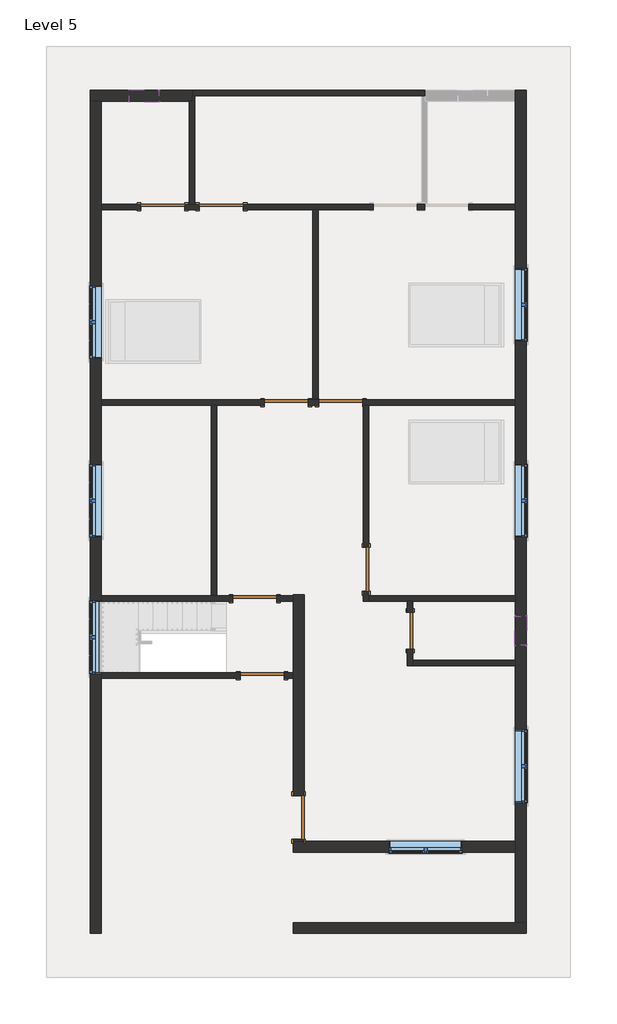
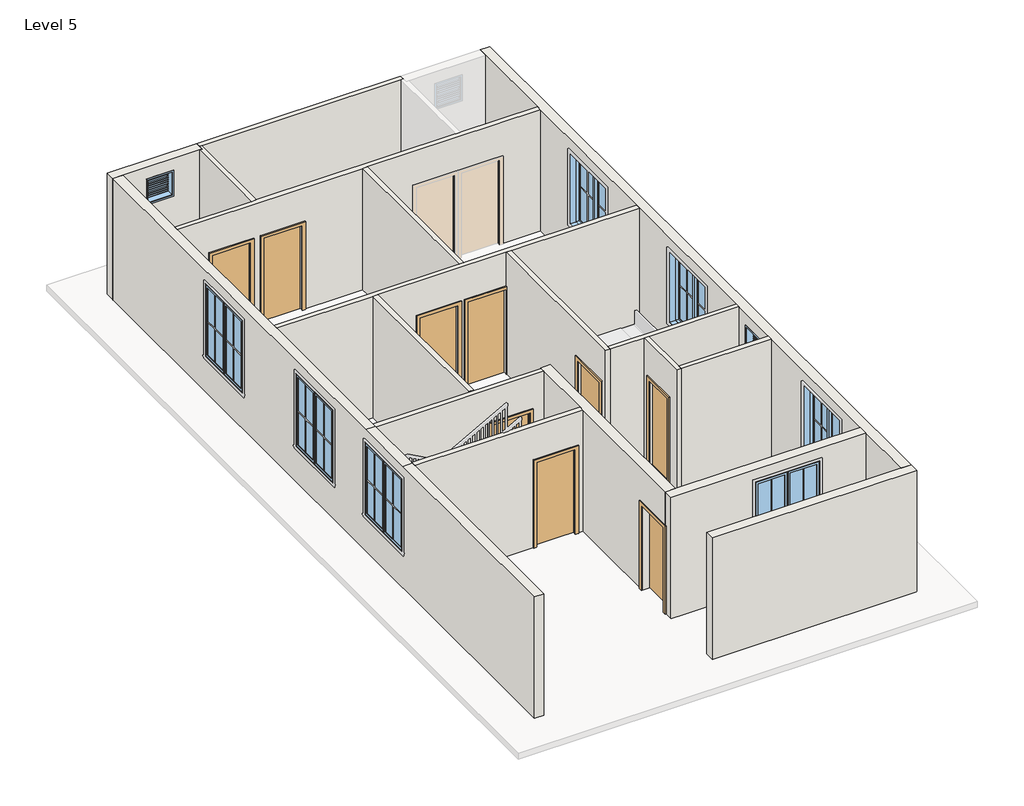
# One storey, part 1 of 3: 18 walls, 9 doors, 9 windows.
"""IFC4 building model written with IfcOpenShell, lengths in millimetres."""

from ifc_helpers import new_model, si_unit, frame, origin, place, context, project, spatial, polyline, outline, extrude, faceted_brep, transform, mapped, element, save
from components import door_78caadf7, single_flush_door_3_e5f9f3c4, single_flush_door_3_305aa2a5, single_flush_door_3_0ca8825f, window_casement_double_win_5_f93960c7, window_f2d8fef0

model = new_model("IFC4")

# Units and contexts
model_context = context("Model", 3, world=origin())
ifc_project = project(units=[si_unit("LENGTHUNIT", "METRE", prefix="MILLI")], contexts=[model_context])

# Site, building, storey
site = spatial("IfcSite", under=ifc_project)
building = spatial("IfcBuilding", under=site)
storey = spatial("IfcBuildingStorey", under=building, Name="Level 5", Elevation=9601.2)

# Doors
placement = place(None, origin())
door_shape = door_78caadf7(model_context)
element("IfcDoor", 1, ObjectType="Single-Flush : DOOR 2'6\"", at=placement, inside=storey, context=model_context, shape_type="MappedRepresentation", body=[
    mapped(door_shape, transform((860.2379845, -2779.6065691, 9601.2), x_axis=(0.0, 1.0, 0.0), y_axis=(-1.0, 0.0, 0.0), z_axis=(0.0, 0.0, 1.0))),
])
single_flush_door_3_shape = single_flush_door_3_e5f9f3c4(model_context)
element("IfcDoor", 2, ObjectType="Single-Flush : DOOR 3'", at=placement, inside=storey, context=model_context, shape_type="MappedRepresentation", body=[
    mapped(single_flush_door_3_shape, transform((-54.1620155, -1503.2565691, 9601.2), x_axis=(0.0, -1.0, 0.0), y_axis=(1.0, 0.0, 0.0), z_axis=(0.0, 0.0, 1.0))),
])
element("IfcDoor", 3, ObjectType="Single-Flush : DOOR 3'", at=placement, inside=storey, context=model_context, shape_type="MappedRepresentation", body=[
    mapped(single_flush_door_3_shape, transform((-1717.8620155, 1963.8434309, 9601.2), x_axis=(1.0, 0.0, 0.0), y_axis=(0.0, 1.0, 0.0), z_axis=(0.0, 0.0, 1.0))),
])
element("IfcDoor", 4, ObjectType="Single-Flush : DOOR 3'", at=placement, inside=storey, context=model_context, shape_type="MappedRepresentation", body=[
    mapped(single_flush_door_3_shape, transform((-2371.9120155, -2112.8565691, 9601.2), x_axis=(1.0, 0.0, 0.0), y_axis=(0.0, 1.0, 0.0), z_axis=(0.0, 0.0, 1.0))),
])
element("IfcDoor", 5, ObjectType="Single-Flush : DOOR 3'", at=placement, inside=storey, context=model_context, shape_type="MappedRepresentation", body=[
    mapped(single_flush_door_3_shape, transform((-2219.5120155, -3713.0565691, 9601.2), x_axis=(1.0, 0.0, 0.0), y_axis=(0.0, 1.0, 0.0), z_axis=(0.0, 0.0, 1.0))),
])
element("IfcDoor", 6, ObjectType="Single-Flush : DOOR 3'", at=placement, inside=storey, context=model_context, shape_type="MappedRepresentation", body=[
    mapped(single_flush_door_3_shape, transform((-4283.2620155, 6040.5434309, 9601.2), x_axis=(1.0, 0.0, 0.0), y_axis=(0.0, 1.0, 0.0), z_axis=(0.0, 0.0, 1.0))),
])
single_flush_door_3_2_shape = single_flush_door_3_305aa2a5(model_context)
element("IfcDoor", 7, ObjectType="Single-Flush : DOOR 3'", at=placement, inside=storey, context=model_context, shape_type="MappedRepresentation", body=[
    mapped(single_flush_door_3_2_shape, transform((-581.2120155, 1963.8434309, 9601.2), x_axis=(-1.0, 0.0, 0.0), y_axis=(0.0, -1.0, 0.0), z_axis=(0.0, 0.0, 1.0))),
])
element("IfcDoor", 8, ObjectType="Single-Flush : DOOR 3'", at=placement, inside=storey, context=model_context, shape_type="MappedRepresentation", body=[
    mapped(single_flush_door_3_2_shape, transform((-3064.0620155, 6040.5434309, 9601.2), x_axis=(-1.0, 0.0, 0.0), y_axis=(0.0, -1.0, 0.0), z_axis=(0.0, 0.0, 1.0))),
])
single_flush_door_3_3_shape = single_flush_door_3_0ca8825f(model_context)
element("IfcDoor", 9, ObjectType="Single-Flush : DOOR 3'", at=placement, inside=storey, context=model_context, shape_type="MappedRepresentation", body=[
    mapped(single_flush_door_3_3_shape, transform((-1457.5120155, -6665.8065691, 9601.2), x_axis=(0.0, -1.0, 0.0), y_axis=(1.0, 0.0, 0.0), z_axis=(0.0, 0.0, 1.0))),
])

# Walls
element("IfcWall", 10, ObjectType="WALL 4.5\"", at=placement, inside=storey, context=model_context, shape_type="Brep", body=[
    faceted_brep([(-3673.6620155, 8345.5934309, 9601.2), (-3616.5120155, 8345.5934309, 9601.2), (1107.8879845, 8345.5934309, 9601.2), (1165.0379845, 8345.5934309, 9601.2), (1165.0379845, 8345.5934309, 12649.2), (1107.8879845, 8345.5934309, 12649.2), (-3616.5120155, 8345.5934309, 12649.2), (-3673.6620155, 8345.5934309, 12649.2), (-3673.6620155, 8459.8934309, 9601.2), (-3673.6620155, 8459.8934309, 12649.2), (1165.0379845, 8459.8934309, 12649.2), (1165.0379845, 8459.8934309, 9601.2)], [[[0, 1, 2, 3, 4, 5, 6, 7]], [[8, 9, 10, 11]], [[3, 2, 1, 0, 8, 11]], [[4, 3, 11, 10]], [[0, 7, 9, 8]], [[7, 6, 5, 4, 10, 9]]]),
])
element("IfcWall", 11, ObjectType="WALL 4.5\"", at=placement, inside=storey, context=model_context, shape_type="SweptSolid", body=[
    extrude(outline(polyline([(-3730.8120155, 6097.6934309), (-3730.8120155, 8231.2934309), (-3673.6620155, 8231.2934309), (-3673.6620155, 8345.5934309), (-3616.5120155, 8345.5934309), (-3616.5120155, 6097.6934309), (-3730.8120155, 6097.6934309)])), frame((0.0, 0.0, 9601.2), z_axis=(0.0, 0.0, 1.0), x_axis=(1.0, 0.0, 0.0)), (0.0, 0.0, 1.0), 3048.0),
])
element("IfcWall", 12, ObjectType="WALL 4.5\"", at=placement, inside=storey, context=model_context, shape_type="Brep", body=[
    faceted_brep([(1165.0379845, 6097.6934309, 11734.8), (1165.0379845, 6097.6934309, 9601.2), (1107.8879845, 6097.6934309, 9601.2), (1012.6379845, 6097.6934309, 9601.2), (1012.6379845, 6097.6934309, 11734.8), (98.2379845, 6097.6934309, 11734.8), (98.2379845, 6097.6934309, 9601.2), (-2606.8620155, 6097.6934309, 9601.2), (-2606.8620155, 6097.6934309, 11734.8), (-3521.2620155, 6097.6934309, 11734.8), (-3521.2620155, 6097.6934309, 9601.2), (-3616.5120155, 6097.6934309, 9601.2), (-3730.8120155, 6097.6934309, 9601.2), (-3826.0620155, 6097.6934309, 9601.2), (-3826.0620155, 6097.6934309, 11734.8), (-4740.4620155, 6097.6934309, 11734.8), (-4740.4620155, 6097.6934309, 9601.2), (-5559.6120155, 6097.6934309, 9601.2), (-5559.6120155, 6097.6934309, 12649.2), (-3730.8120155, 6097.6934309, 12649.2), (-3616.5120155, 6097.6934309, 12649.2), (1107.8879845, 6097.6934309, 12649.2), (1222.1879845, 6097.6934309, 12649.2), (3050.9879845, 6097.6934309, 12649.2), (3050.9879845, 6097.6934309, 9601.2), (2079.4379845, 6097.6934309, 9601.2), (2079.4379845, 6097.6934309, 11734.8), (1012.6379845, 5983.3934309, 9601.2), (1165.0379845, 5983.3934309, 9601.2), (1165.0379845, 5983.3934309, 11734.8), (2079.4379845, 5983.3934309, 11734.8), (2079.4379845, 5983.3934309, 9601.2), (3050.9879845, 5983.3934309, 9601.2), (3050.9879845, 5983.3934309, 12649.2), (-1051.1120155, 5983.3934309, 12649.2), (-1165.4120155, 5983.3934309, 12649.2), (-5559.6120155, 5983.3934309, 12649.2), (-5559.6120155, 5983.3934309, 9601.2), (-4740.4620155, 5983.3934309, 9601.2), (-4740.4620155, 5983.3934309, 11734.8), (-3826.0620155, 5983.3934309, 11734.8), (-3826.0620155, 5983.3934309, 9601.2), (-3521.2620155, 5983.3934309, 9601.2), (-3521.2620155, 5983.3934309, 11734.8), (-2606.8620155, 5983.3934309, 11734.8), (-2606.8620155, 5983.3934309, 9601.2), (-1165.4120155, 5983.3934309, 9601.2), (-1051.1120155, 5983.3934309, 9601.2), (98.2379845, 5983.3934309, 9601.2), (98.2379845, 5983.3934309, 11734.8), (1012.6379845, 5983.3934309, 11734.8)], [[[0, 1, 2, 3, 4, 5, 6, 7, 8, 9, 10, 11, 12, 13, 14, 15, 16, 17, 18, 19, 20, 21, 22, 23, 24, 25, 26]], [[27, 28, 29, 30, 31, 32, 33, 34, 35, 36, 37, 38, 39, 40, 41, 42, 43, 44, 45, 46, 47, 48, 49, 50]], [[38, 37, 17, 16]], [[13, 12, 11, 10, 42, 41]], [[48, 47, 46, 45, 7, 6]], [[25, 24, 32, 31]], [[3, 2, 1, 28, 27]], [[18, 17, 37, 36]], [[24, 23, 33, 32]], [[14, 13, 41, 40]], [[15, 14, 40, 39]], [[16, 15, 39, 38]], [[43, 42, 10, 9]], [[44, 43, 9, 8]], [[45, 44, 8, 7]], [[4, 3, 27, 50]], [[5, 4, 50, 49]], [[6, 5, 49, 48]], [[29, 28, 1, 0]], [[30, 29, 0, 26]], [[31, 30, 26, 25]], [[23, 22, 21, 20, 19, 18, 36, 35, 34, 33]]]),
])
element("IfcWall", 13, ObjectType="WALL 4.5\"", at=placement, inside=storey, context=model_context, shape_type="SweptSolid", body=[
    extrude(outline(polyline([(-1165.4120155, 2020.9934309), (-1165.4120155, 5983.3934309), (-1051.1120155, 5983.3934309), (-1051.1120155, 2020.9934309), (-1165.4120155, 2020.9934309)])), frame((0.0, 0.0, 9601.2), z_axis=(0.0, 0.0, 1.0), x_axis=(1.0, 0.0, 0.0)), (0.0, 0.0, 1.0), 3048.0),
])
element("IfcWall", 14, ObjectType="WALL 4.5\"", at=placement, inside=storey, context=model_context, shape_type="Brep", body=[
    faceted_brep([(-1260.6620155, 1906.6934309, 11734.8), (-1260.6620155, 1906.6934309, 9601.2), (-1038.4120155, 1906.6934309, 9601.2), (-1038.4120155, 1906.6934309, 11734.8), (-124.0120155, 1906.6934309, 11734.8), (-124.0120155, 1906.6934309, 9601.2), (-111.3120155, 1906.6934309, 9601.2), (2.9879845, 1906.6934309, 9601.2), (3050.9879845, 1906.6934309, 9601.2), (3050.9879845, 1906.6934309, 12649.2), (2.9879845, 1906.6934309, 12649.2), (-111.3120155, 1906.6934309, 12649.2), (-3159.3120155, 1906.6934309, 12649.2), (-3273.6120155, 1906.6934309, 12649.2), (-5559.6120155, 1906.6934309, 12649.2), (-5559.6120155, 1906.6934309, 9601.2), (-3273.6120155, 1906.6934309, 9601.2), (-3159.3120155, 1906.6934309, 9601.2), (-2175.0620155, 1906.6934309, 9601.2), (-2175.0620155, 1906.6934309, 11734.8), (-1038.4120155, 2020.9934309, 9601.2), (-1051.1120155, 2020.9934309, 9601.2), (-1165.4120155, 2020.9934309, 9601.2), (-1260.6620155, 2020.9934309, 9601.2), (-1260.6620155, 2020.9934309, 11734.8), (-2175.0620155, 2020.9934309, 11734.8), (-2175.0620155, 2020.9934309, 9601.2), (-5559.6120155, 2020.9934309, 9601.2), (-5559.6120155, 2020.9934309, 12649.2), (-1165.4120155, 2020.9934309, 12649.2), (-1051.1120155, 2020.9934309, 12649.2), (3050.9879845, 2020.9934309, 12649.2), (3050.9879845, 2020.9934309, 9601.2), (-124.0120155, 2020.9934309, 9601.2), (-124.0120155, 2020.9934309, 11734.8), (-1038.4120155, 2020.9934309, 11734.8)], [[[0, 1, 2, 3, 4, 5, 6, 7, 8, 9, 10, 11, 12, 13, 14, 15, 16, 17, 18, 19]], [[20, 21, 22, 23, 24, 25, 26, 27, 28, 29, 30, 31, 32, 33, 34, 35]], [[33, 32, 8, 7, 6, 5]], [[2, 1, 23, 22, 21, 20]], [[18, 17, 16, 15, 27, 26]], [[15, 14, 28, 27]], [[9, 8, 32, 31]], [[3, 2, 20, 35]], [[4, 3, 35, 34]], [[5, 4, 34, 33]], [[24, 23, 1, 0]], [[25, 24, 0, 19]], [[26, 25, 19, 18]], [[14, 13, 12, 11, 10, 9, 31, 30, 29, 28]]]),
])
element("IfcWall", 15, ObjectType="WALL 4.5\"", at=placement, inside=storey, context=model_context, shape_type="SweptSolid", body=[
    extrude(outline(polyline([(-3273.6120155, -2032.8465691), (-3273.6120155, 1906.6934309), (-3159.3120155, 1906.6934309), (-3159.3120155, -2032.8465691), (-3273.6120155, -2032.8465691)])), frame((0.0, 0.0, 9601.2), z_axis=(0.0, 0.0, 1.0), x_axis=(1.0, 0.0, 0.0)), (0.0, 0.0, 1.0), 3048.0),
])
element("IfcWall", 16, ObjectType="WALL 4.5\"", at=placement, inside=storey, context=model_context, shape_type="SweptSolid", body=[
    extrude(outline(polyline([(11734.8, -1914.7120155), (9601.2, -1914.7120155), (9601.2, -1571.8120155), (12649.2, -1571.8120155), (12649.2, -5559.6120155), (9601.2, -5559.6120155), (9601.2, -2829.1120155), (11734.8, -2829.1120155), (11734.8, -1914.7120155)])), frame((0.0, -2170.0065691, 0.0), z_axis=(0.0, 1.0, 0.0), x_axis=(0.0, 0.0, 1.0)), (0.0, 0.0, 1.0), 114.3),
])
element("IfcWall", 17, ObjectType="WALL 4.5\"", at=placement, inside=storey, context=model_context, shape_type="SweptSolid", body=[
    extrude(outline(polyline([(11734.8, -1762.3120155), (9601.2, -1762.3120155), (9601.2, -1571.8120155), (12649.2, -1571.8120155), (12649.2, -5559.6120155), (9601.2, -5559.6120155), (9601.2, -2676.7120155), (11734.8, -2676.7120155), (11734.8, -1762.3120155)])), frame((0.0, -3770.2065691, 0.0), z_axis=(0.0, 1.0, 0.0), x_axis=(0.0, 0.0, 1.0)), (0.0, 0.0, 1.0), 114.3),
])
element("IfcWall", 18, ObjectType="WALL 4.5\"", at=placement, inside=storey, context=model_context, shape_type="Brep", body=[
    faceted_brep([(-111.3120155, -1960.4565691, 11734.8), (-111.3120155, -1960.4565691, 9601.2), (-111.3120155, -2170.0065691, 9601.2), (-111.3120155, -2170.0065691, 12649.2), (-111.3120155, 1906.6934309, 12649.2), (-111.3120155, 1906.6934309, 9601.2), (-111.3120155, -1046.0565691, 9601.2), (-111.3120155, -1046.0565691, 11734.8), (2.9879845, -2170.0065691, 9601.2), (2.9879845, -2055.7065691, 9601.2), (2.9879845, -1960.4565691, 9601.2), (2.9879845, -1960.4565691, 11734.8), (2.9879845, -1046.0565691, 11734.8), (2.9879845, -1046.0565691, 9601.2), (2.9879845, 1906.6934309, 9601.2), (2.9879845, 1906.6934309, 12649.2), (2.9879845, -2055.7065691, 12649.2), (2.9879845, -2170.0065691, 12649.2)], [[[0, 1, 2, 3, 4, 5, 6, 7]], [[8, 9, 10, 11, 12, 13, 14, 15, 16, 17]], [[6, 5, 14, 13]], [[2, 1, 10, 9, 8]], [[5, 4, 15, 14]], [[3, 2, 8, 17]], [[11, 10, 1, 0]], [[12, 11, 0, 7]], [[13, 12, 7, 6]], [[4, 3, 17, 16, 15]]]),
])
element("IfcWall", 19, ObjectType="WALL 4.5\"", at=placement, inside=storey, context=model_context, shape_type="Brep", body=[
    faceted_brep([(2.9879845, -2170.0065691, 9601.2), (803.0879845, -2170.0065691, 9601.2), (917.3879845, -2170.0065691, 9601.2), (3050.9879845, -2170.0065691, 9601.2), (3050.9879845, -2170.0065691, 12649.2), (917.3879845, -2170.0065691, 12649.2), (803.0879845, -2170.0065691, 12649.2), (2.9879845, -2170.0065691, 12649.2), (2.9879845, -2055.7065691, 9601.2), (2.9879845, -2055.7065691, 12649.2), (3050.9879845, -2055.7065691, 12649.2), (3050.9879845, -2055.7065691, 9601.2)], [[[0, 1, 2, 3, 4, 5, 6, 7]], [[8, 9, 10, 11]], [[3, 2, 1, 0, 8, 11]], [[0, 7, 9, 8]], [[4, 3, 11, 10]], [[7, 6, 5, 4, 10, 9]]]),
])
element("IfcWall", 20, ObjectType="WALL 4.5\"", at=placement, inside=storey, context=model_context, shape_type="Brep", body=[
    faceted_brep([(803.0879845, -2170.0065691, 9601.2), (803.0879845, -2398.6065691, 9601.2), (803.0879845, -2398.6065691, 11734.8), (803.0879845, -3160.6065691, 11734.8), (803.0879845, -3160.6065691, 9601.2), (803.0879845, -3503.5065691, 9601.2), (803.0879845, -3503.5065691, 12649.2), (803.0879845, -2170.0065691, 12649.2), (917.3879845, -2398.6065691, 11734.8), (917.3879845, -2398.6065691, 9601.2), (917.3879845, -2170.0065691, 9601.2), (917.3879845, -2170.0065691, 12649.2), (917.3879845, -3389.2065691, 12649.2), (917.3879845, -3503.5065691, 12649.2), (917.3879845, -3503.5065691, 9601.2), (917.3879845, -3389.2065691, 9601.2), (917.3879845, -3160.6065691, 9601.2), (917.3879845, -3160.6065691, 11734.8)], [[[0, 1, 2, 3, 4, 5, 6, 7]], [[8, 9, 10, 11, 12, 13, 14, 15, 16, 17]], [[10, 9, 1, 0]], [[16, 15, 14, 5, 4]], [[0, 7, 11, 10]], [[6, 5, 14, 13]], [[2, 1, 9, 8]], [[3, 2, 8, 17]], [[4, 3, 17, 16]], [[7, 6, 13, 12, 11]]]),
])
element("IfcWall", 21, ObjectType="WALL 4.5\"", at=placement, inside=storey, context=model_context, shape_type="SweptSolid", body=[
    extrude(outline(polyline([(917.3879845, -3389.2065691), (3050.9879845, -3389.2065691), (3050.9879845, -3503.5065691), (917.3879845, -3503.5065691), (917.3879845, -3389.2065691)])), frame((0.0, 0.0, 9601.2), z_axis=(0.0, 0.0, 1.0), x_axis=(1.0, 0.0, 0.0)), (0.0, 0.0, 1.0), 3048.0),
])
element("IfcWall", 22, ObjectType="WALL 9\"", at=placement, inside=storey, context=model_context, shape_type="Brep", body=[
    faceted_brep([(-3673.6620155, 8459.8934309, 9601.2), (-5788.2120155, 8459.8934309, 9601.2), (-5788.2120155, 8459.8934309, 12649.2), (-3673.6620155, 8459.8934309, 12649.2), (-4978.5870155, 8459.8934309, 12344.4), (-4978.5870155, 8459.8934309, 11734.8), (-4368.9870155, 8459.8934309, 11734.8), (-4368.9870155, 8459.8934309, 12344.4), (-3673.6620155, 8231.2934309, 9601.2), (-3673.6620155, 8231.2934309, 12649.2), (-3730.8120155, 8231.2934309, 12649.2), (-5559.6120155, 8231.2934309, 12649.2), (-5788.2120155, 8231.2934309, 12649.2), (-5788.2120155, 8231.2934309, 9601.2), (-5559.6120155, 8231.2934309, 9601.2), (-3730.8120155, 8231.2934309, 9601.2), (-4978.5870155, 8231.2934309, 12344.4), (-4368.9870155, 8231.2934309, 12344.4), (-4368.9870155, 8231.2934309, 11734.8), (-4978.5870155, 8231.2934309, 11734.8), (-3673.6620155, 8345.5934309, 9601.2), (-3673.6620155, 8345.5934309, 12649.2)], [[[0, 1, 2, 3], [4, 5, 6, 7]], [[8, 9, 10, 11, 12, 13, 14, 15], [16, 17, 18, 19]], [[1, 0, 20, 8, 15, 14, 13]], [[0, 3, 21, 9, 8, 20]], [[2, 1, 13, 12]], [[5, 4, 16, 19]], [[6, 5, 19, 18]], [[7, 6, 18, 17]], [[4, 7, 17, 16]], [[3, 2, 12, 11, 10, 9, 21]]]),
])
element("IfcWall", 23, ObjectType="WALL 9\"", at=placement, inside=storey, context=model_context, shape_type="Brep", body=[
    faceted_brep([(-5788.2120155, 8231.2934309, 9601.2), (-5788.2120155, -9078.8065691, 9601.2), (-5788.2120155, -9078.8065691, 12649.2), (-5788.2120155, -3674.9565691, 12649.2), (-5788.2120155, -2150.9565691, 12649.2), (-5788.2120155, 8231.2934309, 12649.2), (-5788.2120155, 4402.2434309, 12344.4), (-5788.2120155, 2878.2434309, 12344.4), (-5788.2120155, 2878.2434309, 10515.6), (-5788.2120155, 4402.2434309, 10515.6), (-5788.2120155, -2150.9565691, 12344.4), (-5788.2120155, -3674.9565691, 12344.4), (-5788.2120155, -3674.9565691, 10515.6), (-5788.2120155, -2150.9565691, 10515.6), (-5788.2120155, 687.4934309, 12344.4), (-5788.2120155, -836.5065691, 12344.4), (-5788.2120155, -836.5065691, 10515.6), (-5788.2120155, 687.4934309, 10515.6), (-5559.6120155, 8231.2934309, 9601.2), (-5559.6120155, 8231.2934309, 12649.2), (-5559.6120155, 6097.6934309, 12649.2), (-5559.6120155, 5983.3934309, 12649.2), (-5559.6120155, 2020.9934309, 12649.2), (-5559.6120155, 1906.6934309, 12649.2), (-5559.6120155, -2055.7065691, 12649.2), (-5559.6120155, -2150.9565691, 12649.2), (-5559.6120155, -2170.0065691, 12649.2), (-5559.6120155, -3655.9065691, 12649.2), (-5559.6120155, -3674.9565691, 12649.2), (-5559.6120155, -3770.2065691, 12649.2), (-5559.6120155, -9078.8065691, 12649.2), (-5559.6120155, -9078.8065691, 9601.2), (-5559.6120155, -3770.2065691, 9601.2), (-5559.6120155, -3655.9065691, 9601.2), (-5559.6120155, -2170.0065691, 9601.2), (-5559.6120155, -2055.7065691, 9601.2), (-5559.6120155, 1906.6934309, 9601.2), (-5559.6120155, 2020.9934309, 9601.2), (-5559.6120155, 5983.3934309, 9601.2), (-5559.6120155, 6097.6934309, 9601.2), (-5559.6120155, 4402.2434309, 12344.4), (-5559.6120155, 4402.2434309, 10515.6), (-5559.6120155, 2878.2434309, 10515.6), (-5559.6120155, 2878.2434309, 12344.4), (-5559.6120155, -2150.9565691, 12344.4), (-5559.6120155, -2150.9565691, 10515.6), (-5559.6120155, -3674.9565691, 10515.6), (-5559.6120155, -3674.9565691, 12344.4), (-5559.6120155, 687.4934309, 12344.4), (-5559.6120155, 687.4934309, 10515.6), (-5559.6120155, -836.5065691, 10515.6), (-5559.6120155, -836.5065691, 12344.4)], [[[0, 1, 2, 3, 4, 5], [6, 7, 8, 9], [10, 11, 12, 13], [14, 15, 16, 17]], [[18, 19, 20, 21, 22, 23, 24, 25, 26, 27, 28, 29, 30, 31, 32, 33, 34, 35, 36, 37, 38, 39], [40, 41, 42, 43], [44, 45, 46, 47], [48, 49, 50, 51]], [[1, 0, 18, 39, 38, 37, 36, 35, 34, 33, 32, 31]], [[2, 1, 31, 30]], [[0, 5, 19, 18]], [[41, 40, 6, 9]], [[42, 41, 9, 8]], [[43, 42, 8, 7]], [[40, 43, 7, 6]], [[45, 44, 10, 13]], [[46, 45, 13, 12]], [[47, 46, 12, 11]], [[44, 47, 11, 10]], [[49, 48, 14, 17]], [[50, 49, 17, 16]], [[51, 50, 16, 15]], [[48, 51, 15, 14]], [[4, 3, 28, 27, 26, 25]], [[3, 2, 30, 29, 28]], [[5, 4, 25, 24, 23, 22, 21, 20, 19]]]),
])
element("IfcWall", 24, ObjectType="WALL 9\"", at=placement, inside=storey, context=model_context, shape_type="Brep", body=[
    faceted_brep([(-1571.8120155, -9078.8065691, 9601.2), (3279.5879845, -9078.8065691, 9601.2), (3279.5879845, -9078.8065691, 12649.2), (-1571.8120155, -9078.8065691, 12649.2), (-1571.8120155, -8850.2065691, 9601.2), (-1571.8120155, -8850.2065691, 12649.2), (3050.9879845, -8850.2065691, 12649.2), (3279.5879845, -8850.2065691, 12649.2), (3279.5879845, -8850.2065691, 9601.2), (3050.9879845, -8850.2065691, 9601.2)], [[[0, 1, 2, 3]], [[4, 5, 6, 7, 8, 9]], [[1, 0, 4, 9, 8]], [[0, 3, 5, 4]], [[2, 1, 8, 7]], [[3, 2, 7, 6, 5]]]),
])
element("IfcWall", 25, ObjectType="WALL 9\"", at=placement, inside=storey, context=model_context, shape_type="Brep", body=[
    faceted_brep([(3279.5879845, -8850.2065691, 9601.2), (3279.5879845, 8459.8934309, 9601.2), (3279.5879845, 8459.8934309, 12649.2), (3279.5879845, -8850.2065691, 12649.2), (3279.5879845, 3240.1934309, 12344.4), (3279.5879845, 4764.1934309, 12344.4), (3279.5879845, 4764.1934309, 10515.6), (3279.5879845, 3240.1934309, 10515.6), (3279.5879845, -836.5065691, 12344.4), (3279.5879845, 687.4934309, 12344.4), (3279.5879845, 687.4934309, 10515.6), (3279.5879845, -836.5065691, 10515.6), (3279.5879845, -6361.0065691, 12344.4), (3279.5879845, -4837.0065691, 12344.4), (3279.5879845, -4837.0065691, 10515.6), (3279.5879845, -6361.0065691, 10515.6), (3279.5879845, -2474.8065691, 12344.4), (3279.5879845, -2474.8065691, 11734.8), (3279.5879845, -3084.4065691, 11734.8), (3279.5879845, -3084.4065691, 12344.4), (3050.9879845, -8850.2065691, 9601.2), (3050.9879845, -8850.2065691, 12649.2), (3050.9879845, -7389.7065691, 12649.2), (3050.9879845, -7161.1065691, 12649.2), (3050.9879845, -3503.5065691, 12649.2), (3050.9879845, -3389.2065691, 12649.2), (3050.9879845, -2170.0065691, 12649.2), (3050.9879845, -2055.7065691, 12649.2), (3050.9879845, 1906.6934309, 12649.2), (3050.9879845, 2020.9934309, 12649.2), (3050.9879845, 5983.3934309, 12649.2), (3050.9879845, 6097.6934309, 12649.2), (3050.9879845, 8231.2934309, 12649.2), (3050.9879845, 8459.8934309, 12649.2), (3050.9879845, 8459.8934309, 9601.2), (3050.9879845, 8231.2934309, 9601.2), (3050.9879845, 6097.6934309, 9601.2), (3050.9879845, 5983.3934309, 9601.2), (3050.9879845, 2020.9934309, 9601.2), (3050.9879845, 1906.6934309, 9601.2), (3050.9879845, -2055.7065691, 9601.2), (3050.9879845, -2170.0065691, 9601.2), (3050.9879845, -3389.2065691, 9601.2), (3050.9879845, -3503.5065691, 9601.2), (3050.9879845, -7161.1065691, 9601.2), (3050.9879845, -7389.7065691, 9601.2), (3050.9879845, 3240.1934309, 12344.4), (3050.9879845, 3240.1934309, 10515.6), (3050.9879845, 4764.1934309, 10515.6), (3050.9879845, 4764.1934309, 12344.4), (3050.9879845, -836.5065691, 12344.4), (3050.9879845, -836.5065691, 10515.6), (3050.9879845, 687.4934309, 10515.6), (3050.9879845, 687.4934309, 12344.4), (3050.9879845, -6361.0065691, 12344.4), (3050.9879845, -6361.0065691, 10515.6), (3050.9879845, -4837.0065691, 10515.6), (3050.9879845, -4837.0065691, 12344.4), (3050.9879845, -2474.8065691, 12344.4), (3050.9879845, -3084.4065691, 12344.4), (3050.9879845, -3084.4065691, 11734.8), (3050.9879845, -2474.8065691, 11734.8)], [[[0, 1, 2, 3], [4, 5, 6, 7], [8, 9, 10, 11], [12, 13, 14, 15], [16, 17, 18, 19]], [[20, 21, 22, 23, 24, 25, 26, 27, 28, 29, 30, 31, 32, 33, 34, 35, 36, 37, 38, 39, 40, 41, 42, 43, 44, 45], [46, 47, 48, 49], [50, 51, 52, 53], [54, 55, 56, 57], [58, 59, 60, 61]], [[1, 0, 20, 45, 44, 43, 42, 41, 40, 39, 38, 37, 36, 35, 34]], [[0, 3, 21, 20]], [[2, 1, 34, 33]], [[47, 46, 4, 7]], [[48, 47, 7, 6]], [[49, 48, 6, 5]], [[46, 49, 5, 4]], [[51, 50, 8, 11]], [[52, 51, 11, 10]], [[53, 52, 10, 9]], [[50, 53, 9, 8]], [[55, 54, 12, 15]], [[56, 55, 15, 14]], [[57, 56, 14, 13]], [[54, 57, 13, 12]], [[17, 16, 58, 61]], [[18, 17, 61, 60]], [[19, 18, 60, 59]], [[16, 19, 59, 58]], [[3, 2, 33, 32, 31, 30, 29, 28, 27, 26, 25, 24, 23, 22, 21]]]),
])
element("IfcWall", 26, ObjectType="WALL 9\"", at=placement, inside=storey, context=model_context, shape_type="Brep", body=[
    faceted_brep([(3050.9879845, -7161.1065691, 9601.2), (-1343.2120155, -7161.1065691, 9601.2), (-1571.8120155, -7161.1065691, 9601.2), (-1571.8120155, -7161.1065691, 12649.2), (-1343.2120155, -7161.1065691, 12649.2), (3050.9879845, -7161.1065691, 12649.2), (422.0879845, -7161.1065691, 12344.4), (422.0879845, -7161.1065691, 10515.6), (1946.0879845, -7161.1065691, 10515.6), (1946.0879845, -7161.1065691, 12344.4), (3050.9879845, -7389.7065691, 9601.2), (3050.9879845, -7389.7065691, 12649.2), (-1571.8120155, -7389.7065691, 12649.2), (-1571.8120155, -7389.7065691, 9601.2), (422.0879845, -7389.7065691, 12344.4), (1946.0879845, -7389.7065691, 12344.4), (1946.0879845, -7389.7065691, 10515.6), (422.0879845, -7389.7065691, 10515.6)], [[[0, 1, 2, 3, 4, 5], [6, 7, 8, 9]], [[10, 11, 12, 13], [14, 15, 16, 17]], [[2, 1, 0, 10, 13]], [[0, 5, 11, 10]], [[3, 2, 13, 12]], [[7, 6, 14, 17]], [[8, 7, 17, 16]], [[9, 8, 16, 15]], [[6, 9, 15, 14]], [[5, 4, 3, 12, 11]]]),
])
element("IfcWall", 27, ObjectType="WALL 9\"", at=placement, inside=storey, context=model_context, shape_type="Brep", body=[
    faceted_brep([(-1343.2120155, -7161.1065691, 9601.2), (-1343.2120155, -7123.0065691, 9601.2), (-1343.2120155, -7123.0065691, 11734.8), (-1343.2120155, -6208.6065691, 11734.8), (-1343.2120155, -6208.6065691, 9601.2), (-1343.2120155, -2032.8465691, 9601.2), (-1343.2120155, -2032.8465691, 12649.2), (-1343.2120155, -7161.1065691, 12649.2), (-1571.8120155, -7123.0065691, 11734.8), (-1571.8120155, -7123.0065691, 9601.2), (-1571.8120155, -7161.1065691, 9601.2), (-1571.8120155, -7161.1065691, 12649.2), (-1571.8120155, -3770.2065691, 12649.2), (-1571.8120155, -3655.9065691, 12649.2), (-1571.8120155, -2170.0065691, 12649.2), (-1571.8120155, -2055.7065691, 12649.2), (-1571.8120155, -2032.8465691, 12649.2), (-1571.8120155, -2032.8465691, 9601.2), (-1571.8120155, -2055.7065691, 9601.2), (-1571.8120155, -2170.0065691, 9601.2), (-1571.8120155, -3655.9065691, 9601.2), (-1571.8120155, -3770.2065691, 9601.2), (-1571.8120155, -6208.6065691, 9601.2), (-1571.8120155, -6208.6065691, 11734.8)], [[[0, 1, 2, 3, 4, 5, 6, 7]], [[8, 9, 10, 11, 12, 13, 14, 15, 16, 17, 18, 19, 20, 21, 22, 23]], [[10, 9, 1, 0]], [[22, 21, 20, 19, 18, 17, 5, 4]], [[6, 5, 17, 16]], [[0, 7, 11, 10]], [[2, 1, 9, 8]], [[3, 2, 8, 23]], [[4, 3, 23, 22]], [[7, 6, 16, 15, 14, 13, 12, 11]]]),
])

# Windows
window_casement_double_win_5_shape = window_casement_double_win_5_f93960c7(model_context)
element("IfcWindow", 28, ObjectType="Window-Casement-Double : WIN 5'", at=placement, inside=storey, context=model_context, shape_type="MappedRepresentation", body=[
    mapped(window_casement_double_win_5_shape, transform((-5673.9120155, 3640.2434309, 9601.2), x_axis=(0.0, 1.0, 0.0), y_axis=(-1.0, 0.0, 0.0), z_axis=(0.0, 0.0, 1.0))),
])
element("IfcWindow", 29, ObjectType="Window-Casement-Double : WIN 5'", at=placement, inside=storey, context=model_context, shape_type="MappedRepresentation", body=[
    mapped(window_casement_double_win_5_shape, transform((3165.2879845, 4002.1934309, 9601.2), x_axis=(0.0, -1.0, 0.0), y_axis=(1.0, 0.0, 0.0), z_axis=(0.0, 0.0, 1.0))),
])
element("IfcWindow", 30, ObjectType="Window-Casement-Double : WIN 5'", at=placement, inside=storey, context=model_context, shape_type="MappedRepresentation", body=[
    mapped(window_casement_double_win_5_shape, transform((3165.2879845, -74.5065691, 9601.2), x_axis=(0.0, -1.0, 0.0), y_axis=(1.0, 0.0, 0.0), z_axis=(0.0, 0.0, 1.0))),
])
element("IfcWindow", 31, ObjectType="Window-Casement-Double : WIN 5'", at=placement, inside=storey, context=model_context, shape_type="MappedRepresentation", body=[
    mapped(window_casement_double_win_5_shape, transform((3165.2879845, -5599.0065691, 9601.2), x_axis=(0.0, -1.0, 0.0), y_axis=(1.0, 0.0, 0.0), z_axis=(0.0, 0.0, 1.0))),
])
element("IfcWindow", 32, ObjectType="Window-Casement-Double : WIN 5'", at=placement, inside=storey, context=model_context, shape_type="MappedRepresentation", body=[
    mapped(window_casement_double_win_5_shape, transform((1184.0879845, -7275.4065691, 9601.2), x_axis=(-1.0, 0.0, 0.0), y_axis=(0.0, -1.0, 0.0), z_axis=(0.0, 0.0, 1.0))),
])
element("IfcWindow", 33, ObjectType="Window-Casement-Double : WIN 5'", at=placement, inside=storey, context=model_context, shape_type="MappedRepresentation", body=[
    mapped(window_casement_double_win_5_shape, transform((-5673.9120155, -2912.9565691, 9601.2), x_axis=(0.0, 1.0, 0.0), y_axis=(-1.0, 0.0, 0.0), z_axis=(0.0, 0.0, 1.0))),
])
element("IfcWindow", 34, ObjectType="Window-Casement-Double : WIN 5'", at=placement, inside=storey, context=model_context, shape_type="MappedRepresentation", body=[
    mapped(window_casement_double_win_5_shape, transform((-5673.9120155, -74.5065691, 9601.2), x_axis=(0.0, 1.0, 0.0), y_axis=(-1.0, 0.0, 0.0), z_axis=(0.0, 0.0, 1.0))),
])
window_shape = window_f2d8fef0(model_context)
element("IfcWindow", 35, ObjectType="Window-Louvers : 24\" x 24\"", at=placement, inside=storey, context=model_context, shape_type="MappedRepresentation", body=[
    mapped(window_shape, transform((-4673.7870155, 8351.9434309, 10820.4), x_axis=(1.0, 0.0, 0.0), y_axis=(0.0, 1.0, 0.0), z_axis=(0.0, 0.0, 1.0))),
])
element("IfcWindow", 36, ObjectType="Window-Louvers : 24\" x 24\"", at=placement, inside=storey, context=model_context, shape_type="MappedRepresentation", body=[
    mapped(window_shape, transform((3171.6379845, -2779.6065691, 10820.4), x_axis=(0.0, -1.0, 0.0), y_axis=(1.0, 0.0, 0.0), z_axis=(0.0, 0.0, 1.0))),
])

save(model, "model.ifc")

# Revit data of these elements
# Type "Single-Flush : DOOR 2'6\""
#   Type Mark = "10"
#   Construction Type Id = "MDOOR"
#   Assembly Code = "C1020"
#   Analytic Construction = "Metal"
#   Thickness = 0' - 2"
#   Heat Transfer Coefficient (U) = 0.651978 BTU/(h·ft²·°F)
#   Height = 7' - 0"
#   Trim Projection Ext = 0' - 1"
#   Trim Projection Int = 0' - 1"
#   Trim Width = 0' - 3"
#   Width = 2' - 6"
#   Define Thermal Properties by = 1
#   Door Material = Door - Panel
#   Frame Material = Door - Frame
#   Visual Light Transmittance = 0
#   Solar Heat Gain Coefficient = 0
#   Function = (empty or 0)
#   Wall Closure = (empty or 0)
# Type "Single-Flush : DOOR 3'"
#   Type Mark = "9"
#   Construction Type Id = "MDOOR"
#   Assembly Code = "C1020"
#   Analytic Construction = "Metal"
#   Thickness = 0' - 2"
#   Heat Transfer Coefficient (U) = 0.651978 BTU/(h·ft²·°F)
#   Height = 7' - 0"
#   Trim Projection Ext = 0' - 1"
#   Trim Projection Int = 0' - 1"
#   Trim Width = 0' - 3"
#   Width = 3' - 0"
#   Define Thermal Properties by = 1
#   Door Material = Door - Panel
#   Frame Material = Door - Frame
#   Visual Light Transmittance = 0
#   Solar Heat Gain Coefficient = 0
#   Function = (empty or 0)
#   Wall Closure = (empty or 0)
# Type "WALL 4.5\""
#   Assembly Code = "B2010"
#   Layers, outside or top first: 0' - 4 1/2" no material (function 1)
# Type "WALL 9\""
#   Assembly Code = "B2010"
#   Layers, outside or top first: 0' - 9" no material (function 1)
# Type "Window-Casement-Double : WIN 5'"
#   Type Mark = "18"
#   Fire Rating = "0.5h"
#   Assembly Code = "B2020100"
#   Analytic Construction = "Double glazing - domestic"
#   Frame Extension [instance default] = 0' - 0 1/4"
#   Window Inset [instance default] = 0' - 0"
#   Wall Thickness [instance default] = 0' - 6"
#   Interior Wall Closure [instance default] = 0' - 2 1/4"
#   Half Width = 2' - 6"
#   Visual Light Transmittance = 0.81
#   Thermal Resistance (R) = 1.8146 (h·ft²·°F)/BTU
#   Solar Heat Gain Coefficient = 0.76
#   Rough Width = 5' - 0 1/2"
#   Rough Height = 6' - 0 1/2"
#   Height = 6' - 0"
#   Heat Transfer Coefficient (U) = 0.5511 BTU/(h·ft²·°F)
#   Exterior Wall Closure [instance default] = 0' - 1 1/4"
#   Extension Jamb [instance default] = 0' - 2 1/4"
#   Default Sill Height = 3' - 0"
#   Width = 5' - 0"
#   Muntin Visibility = yes
#   Interior Trim Visibility [instance default] = yes
#   Exterior Trim Visibility [instance default] = yes
#   Extension Jamb Visibility [instance default] = yes
#   Interior Trim Material = Wood - Stained
#   Muntin Pattern = Muntin Pattern_2x2 : Muntin Pattern_2x2
#   Interior Trim = Trim-Window-Interior-Flat : Picture Frame
#   Interior Frame Material = Wood - Stained
#   Glass Panel Material = Glass
#   Exterior Trim Material = Clad - White
#   Exterior Trim = Trim-Window-Exterior-Flat : with Sill
#   Exterior Frame Material = Clad - White
#   Wall Closure = (empty or 0)
# Type "Window-Louvers : 24\" x 24\""
#   Type Mark = "19"
#   Construction Type Id = "GSP4R"
#   Assembly Code = "B20"
#   Analytic Construction = "1/8 in Pilkington single glazing"
#   Visual Light Transmittance = 0.9
#   Thermal Resistance (R) = 1.53941 (h·ft²·°F)/BTU
#   Solar Heat Gain Coefficient = 0.78
#   Max Height = 1' - 11.74264"
#   Height = 2' - 0"
#   Heat Transfer Coefficient (U) = 0.6496 BTU/(h·ft²·°F)
#   Blade Width [instance default] = 1' - 10 1/2"
#   Blade Vertical Thickness = 0' - 0.35355"
#   Blade Thickness = 0' - 0 1/4"
#   Blade Spacing = 0' - 1 1/2"
#   Blade Height = 0' - 1.85355"
#   Blade Depth = 0' - 3"
#   Blade Angle = 45.00°
#   Default Sill Height = 3' - 0"
#   Trim Projection_Exterior = 0' - 0 1/2"
#   Trim Projection_Interior = 0' - 0 1/2"
#   Trim Width_Exterior = 0' - 1 1/2"
#   Trim Width_Interior = 0' - 1 1/2"
#   Width = 2' - 0"
#   Max Blade Count = 12
#   Define Thermal Properties by = 1
#   Blade Count = 12
#   Frame Material = Birch
#   Louver Material = Birch
#   Trim Exterior Material = Birch
#   Trim Interior Material = Birch
#   Wall Closure = (empty or 0)
# Element 1 (IfcDoor, "Single-Flush : DOOR 2'6\"")
#   Phase Created = New Construction
#   Materials on its faces: "Door - Frame", "Door - Panel"
# Elements 2, 3, 4, 5, 6, 7, 8, 9 (IfcDoor, "Single-Flush : DOOR 3'")
#   Phase Created = New Construction
#   Materials on its faces: "Door - Frame", "Door - Panel"
# Elements 10, 17 (IfcWall, "WALL 4.5\"")
#   Top Offset = 0' - 0"
#   Base Offset = 0' - 0"
#   Unconnected Height = 10' - 0"
#   wall height = 10' - 0"
#   Phase Created = New Construction
#   Base Constraint = Level 5
#   Materials on its faces: "Default Wall", "Brick, Common"
# Elements 11, 12, 13, 14, 15, 16, 18, 19, 20, 21 (IfcWall, "WALL 4.5\"")
#   Top Offset = 0' - 0"
#   Base Offset = 0' - 0"
#   Unconnected Height = 10' - 0"
#   wall height = 10' - 0"
#   Phase Created = New Construction
#   Base Constraint = Level 5
#   Materials on its faces: "Default Wall"
# Elements 22, 23, 24, 25, 26, 27 (IfcWall, "WALL 9\"")
#   Top Offset = 0' - 0"
#   Base Offset = 0' - 0"
#   Unconnected Height = 10' - 0"
#   wall height = 10' - 0"
#   Phase Created = New Construction
#   Base Constraint = Level 5
#   Materials on its faces: "Default Wall", "Brick, Common"
# Element 28 (IfcWindow, "Window-Casement-Double : WIN 5'")
#   Mark = "31"
#   Window Inset = 0' - 0"
#   Interior Wall Closure = 0' - 2 1/4"
#   Frame Extension = 0' - 0 1/4"
#   Exterior Wall Closure = 0' - 1 1/4"
#   Interior Trim Visibility = yes
#   Exterior Trim Visibility = yes
#   Phase Created = New Construction
#   Materials on its faces: "Wood - Stained", "Glass", "Clad - White"
# Element 29 (IfcWindow, "Window-Casement-Double : WIN 5'")
#   Mark = "32"
#   Window Inset = 0' - 0"
#   Interior Wall Closure = 0' - 2 1/4"
#   Frame Extension = 0' - 0 1/4"
#   Exterior Wall Closure = 0' - 1 1/4"
#   Interior Trim Visibility = yes
#   Exterior Trim Visibility = yes
#   Phase Created = New Construction
#   Materials on its faces: "Wood - Stained", "Glass", "Clad - White"
# Element 30 (IfcWindow, "Window-Casement-Double : WIN 5'")
#   Mark = "33"
#   Window Inset = 0' - 0"
#   Interior Wall Closure = 0' - 2 1/4"
#   Frame Extension = 0' - 0 1/4"
#   Exterior Wall Closure = 0' - 1 1/4"
#   Interior Trim Visibility = yes
#   Exterior Trim Visibility = yes
#   Phase Created = New Construction
#   Materials on its faces: "Wood - Stained", "Glass", "Clad - White"
# Element 31 (IfcWindow, "Window-Casement-Double : WIN 5'")
#   Mark = "34"
#   Window Inset = 0' - 0"
#   Interior Wall Closure = 0' - 2 1/4"
#   Frame Extension = 0' - 0 1/4"
#   Exterior Wall Closure = 0' - 1 1/4"
#   Interior Trim Visibility = yes
#   Exterior Trim Visibility = yes
#   Phase Created = New Construction
#   Materials on its faces: "Wood - Stained", "Glass", "Clad - White"
# Element 32 (IfcWindow, "Window-Casement-Double : WIN 5'")
#   Mark = "35"
#   Window Inset = 0' - 0"
#   Interior Wall Closure = 0' - 2 1/4"
#   Frame Extension = 0' - 0 1/4"
#   Exterior Wall Closure = 0' - 1 1/4"
#   Interior Trim Visibility = yes
#   Exterior Trim Visibility = yes
#   Phase Created = New Construction
#   Materials on its faces: "Wood - Stained", "Glass", "Clad - White"
# Element 33 (IfcWindow, "Window-Casement-Double : WIN 5'")
#   Mark = "36"
#   Window Inset = 0' - 0"
#   Interior Wall Closure = 0' - 2 1/4"
#   Frame Extension = 0' - 0 1/4"
#   Exterior Wall Closure = 0' - 1 1/4"
#   Interior Trim Visibility = yes
#   Exterior Trim Visibility = yes
#   Phase Created = New Construction
#   Materials on its faces: "Wood - Stained", "Glass", "Clad - White"
# Element 34 (IfcWindow, "Window-Casement-Double : WIN 5'")
#   Mark = "37"
#   Window Inset = 0' - 0"
#   Interior Wall Closure = 0' - 2 1/4"
#   Frame Extension = 0' - 0 1/4"
#   Exterior Wall Closure = 0' - 1 1/4"
#   Interior Trim Visibility = yes
#   Exterior Trim Visibility = yes
#   Phase Created = New Construction
#   Materials on its faces: "Wood - Stained", "Glass", "Clad - White"
# Element 35 (IfcWindow, "Window-Louvers : 24\" x 24\"")
#   Mark = "38"
#   Blade Width = 1' - 10 1/2"
#   Phase Created = New Construction
#   Materials on its faces: "Birch"
# Element 36 (IfcWindow, "Window-Louvers : 24\" x 24\"")
#   Mark = "40"
#   Blade Width = 1' - 10 1/2"
#   Phase Created = New Construction
#   Materials on its faces: "Birch"
# Materials
#   "Door - Panel": class "Wood", colour RGB 210 159 95, transparency 0, Cost = 0
#   "Door - Frame": colour RGB 118 70 51, transparency 0, Cost = 0
#   "Wood - Stained": class "Wood", colour RGB 224 178 126, transparency 0, Cost = 0
#   "Glass": class "Glass", colour RGB 0 128 192, transparency 0.75, Description = "Soda Lime Glass", Cost = 0
#   "Clad - White": class "Wood", colour RGB 242 242 238, transparency 0, Cost = 0
#   "Birch": class "Wood", colour RGB 224 178 126, transparency 0, Description = "Betula Alleghaniensis", Cost = 0
#   "Default Wall": colour RGB 128 128 128, transparency 0, Cost = 0
#   "Brick, Common": class "Masonry", colour RGB 170 98 104, transparency 0, Description = "Common brick", Cost = 0
